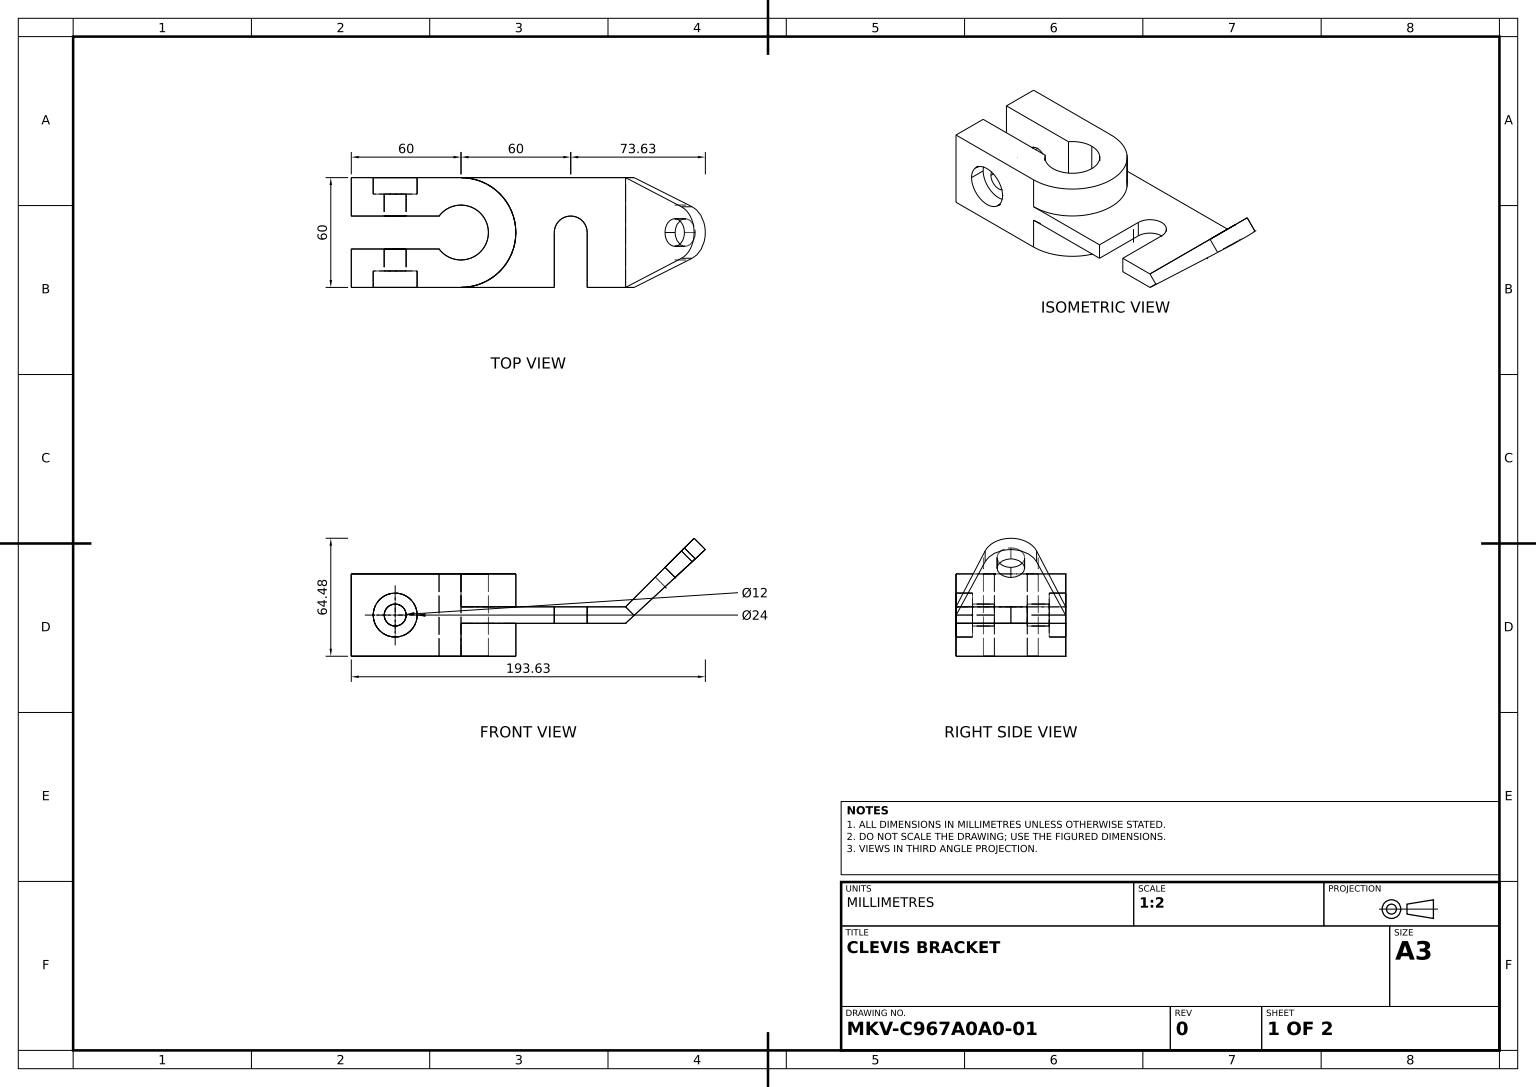
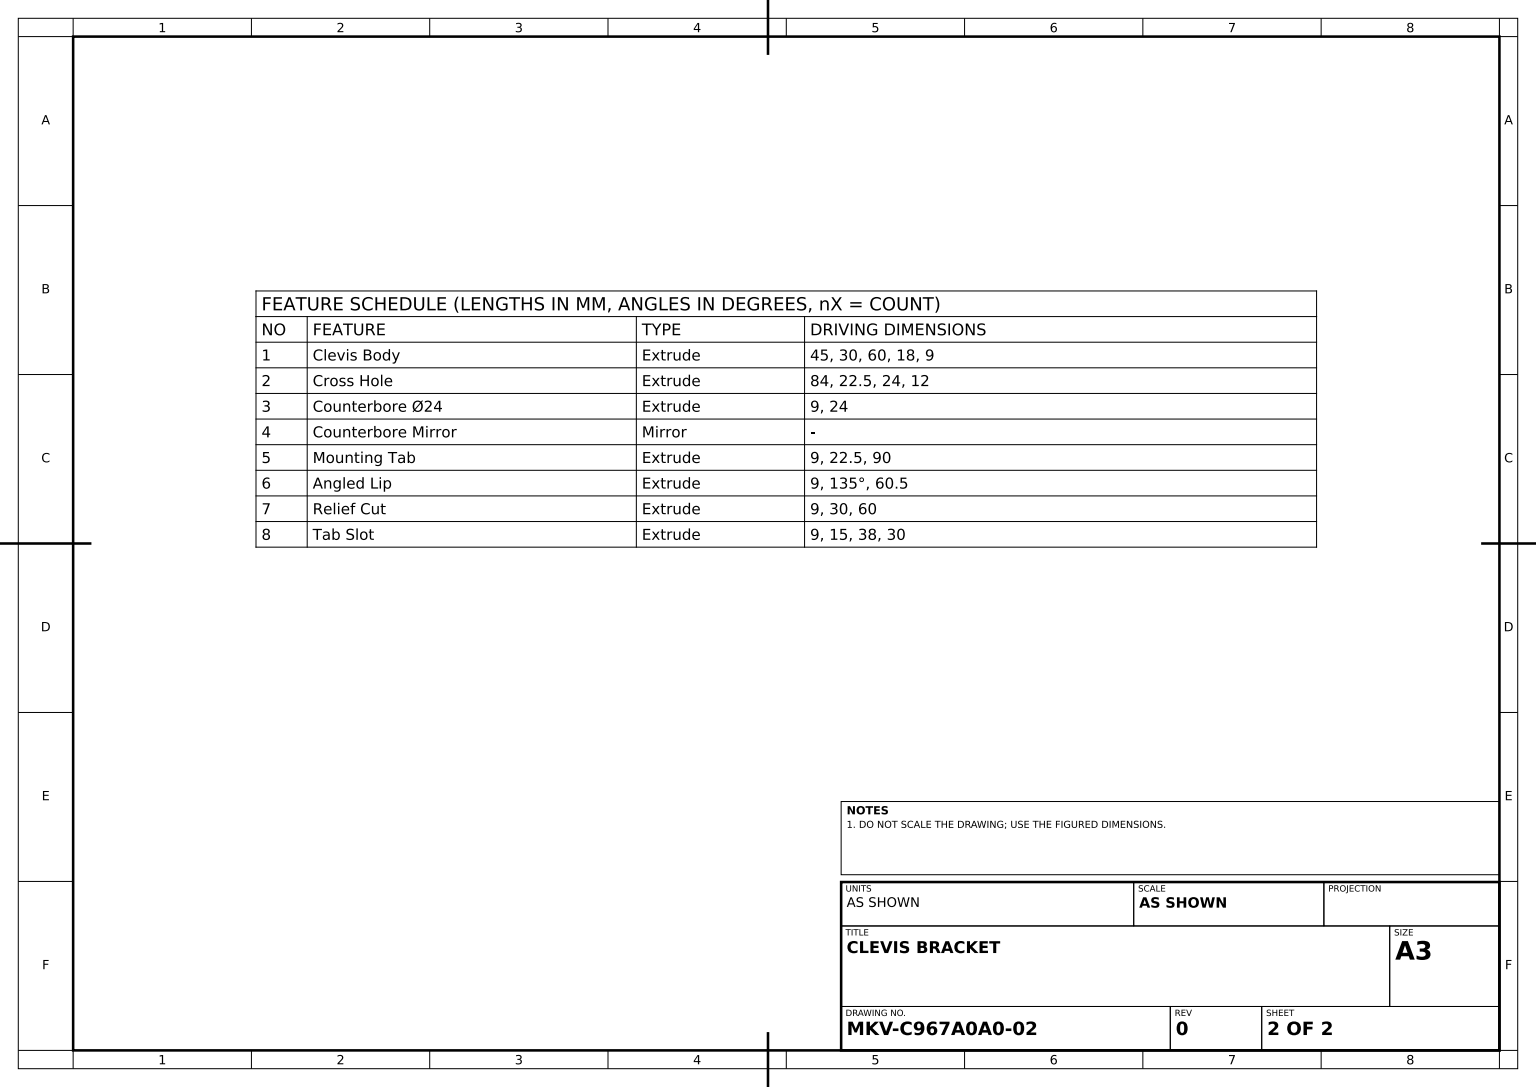
from build123d import *

# Parameters (mm, degrees)
CLEVIS_BODY_DEPTH    = 22.5
CROSS_HOLE_SKETCH_R  = 6
CROSS_HOLE_DEPTH     = 84
COUNTERBORE_SKETCH_R = 12
COUNTERBORE_24_DEPTH = 9
MOUNTING_START       = -22.5
MOUNTING_TAB_DEPTH   = 4.5
ANGLED_LIP_DEPTH     = 60
RELIEF_CUT_DEPTH     = 9
TAB_SLOT_SKETCH_R    = 7.5
TAB_SLOT_DEPTH       = 9


with BuildPart() as part:
    # Clevis Body Sketch → Clevis Body (new, symmetric)
    with BuildSketch(Plane(origin=(0, 0, 0), x_dir=(1, 0, 0), z_dir=(0, 1, 0))):
        with BuildLine():
            Line((-12, 9), (-60, 9))
            Line((-60, 9), (-60, 30))
            Line((-60, 30), (0, 30))
            ThreePointArc((0, 30), (30, 0), (0, -30))
            Line((0, -30), (-60, -30))
            Line((-60, -30), (-60, -9))
            Line((-60, -9), (-12, -9))
            ThreePointArc((-12, -9), (15, 0), (-12, 9))
        make_face()
    extrude(amount=CLEVIS_BODY_DEPTH, both=True)

    # Cross Hole Sketch → Cross Hole (cut)
    with BuildSketch(Plane.XY.offset(30)):
        with Locations((-36, 0)):
            Circle(CROSS_HOLE_SKETCH_R)
    extrude(amount=-CROSS_HOLE_DEPTH, mode=Mode.SUBTRACT)

    # Counterbore Sketch → Counterbore Ø24 (cut)
    with BuildSketch(Plane.XY.offset(30)):
        with Locations((-36, 0)):
            Circle(COUNTERBORE_SKETCH_R)
    counterbore_24 = extrude(amount=-COUNTERBORE_24_DEPTH, mode=Mode.SUBTRACT)

    # Counterbore Mirror: Counterbore Ø24 across plane
    add(counterbore_24.mirror(Plane.XY), mode=Mode.SUBTRACT)

    # Mounting Tab Sketch → Mounting Tab (add, symmetric)
    with BuildSketch(Plane(origin=(0, 22.5, 0), x_dir=(1, 0, 0), z_dir=(0, 1, 0)).offset(MOUNTING_START)):
        with BuildLine():
            Line((0, 30), (90, 30))
            Line((90, 30), (90, -30))
            Line((90, -30), (0, -30))
            ThreePointArc((0, -30), (30, 0), (0, 30))
        make_face()
    extrude(amount=MOUNTING_TAB_DEPTH, both=True)

    # Angled Lip Sketch → Angled Lip (add)
    with BuildSketch(Plane.XY.offset(30)):
        Polygon((90, -4.5), (90, 4.5), (132.779960262, 47.279960262), (139.143921292, 40.915999231), align=None)
    extrude(amount=-ANGLED_LIP_DEPTH)

    # Relief Cut Sketch → Relief Cut (cut)
    with BuildSketch(Plane(origin=(0, 4.5, 0), x_dir=(1, 0, 0), z_dir=(0, 1, 0))):
        with BuildLine():
            Line((51, -30), (51, 0))
            ThreePointArc((51, 0), (60, 9), (69, 0))
            Line((69, 0), (69, -30))
            Line((69, -30), (51, -30))
        make_face()
    extrude(amount=-RELIEF_CUT_DEPTH, mode=Mode.SUBTRACT)

    # Tab Slot Sketch → Tab Slot (cut)
    with BuildSketch(Plane(origin=(42.75, -42.75, 0), x_dir=(0, 0, 1), z_dir=(-0.7071067811865488, 0.7071067811865464, 0))):
        with Locations(Location((0, 104.821590822, 0), (0, 0, 270))):
            Circle(TAB_SLOT_SKETCH_R)
        with BuildLine():
            Line((-30, 66.821590822), (-14.073626439, 110.011295906))
            ThreePointArc((-14.073626439, 110.011295906), (0, 119.821590822), (14.073626439, 110.011295906))
            Line((14.073626439, 110.011295906), (30, 66.821590822))
            Line((30, 66.821590822), (30, 127.321590822))
            Line((30, 127.321590822), (-30, 127.321590822))
            Line((-30, 127.321590822), (-30, 66.821590822))
        make_face()
    extrude(amount=-TAB_SLOT_DEPTH, mode=Mode.SUBTRACT)


solid = part.part
